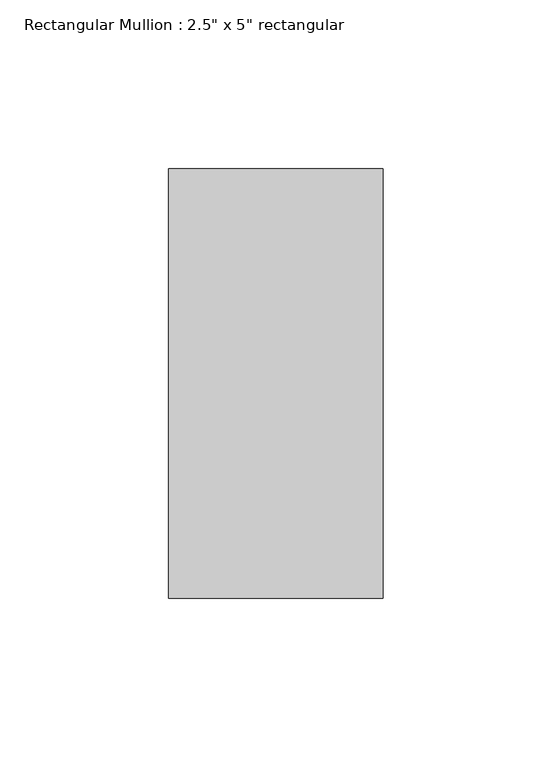
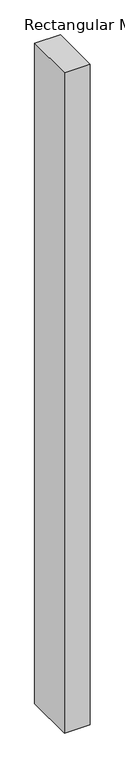
"""IFC4 building model written with IfcOpenShell, lengths in millimetres: member geometry."""

from ifc_helpers import new_model, si_unit, frame, origin, place, context, project, spatial, polyline, outline, extrude, source, transform, mapped, element, save


def member_70523b0d(model_context):
    return source(origin(), model_context, "Body", "SweptSolid", [
        extrude(outline(polyline([(0.0, 63.5), (0.0, -63.5), (-63.5, -63.5), (-63.5, 63.5), (0.0, 63.5)])), frame((0.0, 0.0, -1725.9311114), z_axis=(0.0, 0.0, 1.0), x_axis=(1.0, 0.0, 0.0)), (0.0, 0.0, 1.0), 1725.9311114),
    ])


if __name__ == "__main__":
    model = new_model("IFC4")
    model_context = context("Model", 3, world=origin())
    ifc_project = project(units=[si_unit("LENGTHUNIT", "METRE", prefix="MILLI")], contexts=[model_context])
    site = spatial("IfcSite", under=ifc_project)
    building = spatial("IfcBuilding", under=site)
    placement = place(None, origin())
    member_shape = member_70523b0d(model_context)
    element("IfcMember", 1, ObjectType="Rectangular Mullion : 2.5\" x 5\" rectangular", at=placement, inside=building, context=model_context, shape_type="MappedRepresentation", body=[
        mapped(member_shape, transform((0.0, 0.0, 0.0), x_axis=(1.0, 0.0, 0.0), y_axis=(0.0, 1.0, 0.0), z_axis=(0.0, 0.0, 1.0))),
    ])
    save(model, "model.ifc")

# Revit data of these elements
# Type "Rectangular Mullion : 2.5\" x 5\" rectangular"
#   built-in parameter 1007304 = 0.416667 (stored number, unit not read)
#   built-in parameter 1007301 = 0.104167 (stored number, unit not read)
#   built-in parameter 1007300 = 0.104167 (stored number, unit not read)
# Element 1 (IfcMember, "Rectangular Mullion : 2.5\" x 5\" rectangular")
#   Materials on its faces: "Aluminum"
# Materials
#   "Aluminum": class "Metal", colour RGB 247 247 247, transparency 0, Description = "Aluminum 6061", Cost = 0
